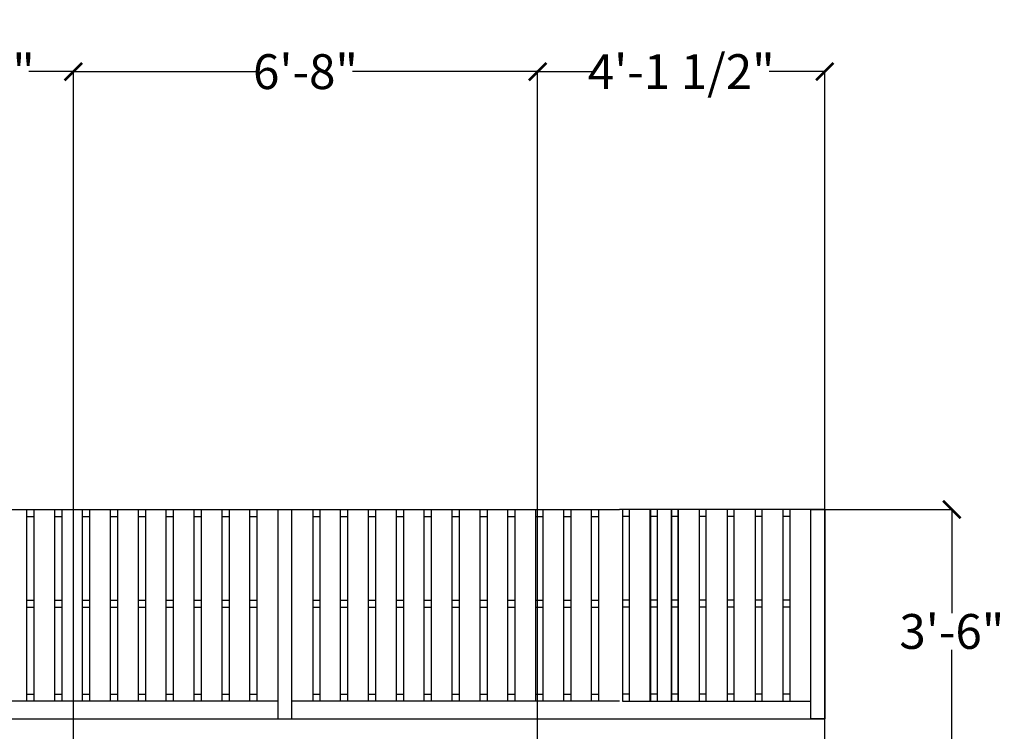
# Model space of a CAD drawing. Units: inches. Extents: x 2278 to 7495, y -71 to 1198.
# Tile 38 of 44: x 5007 to 5177, y 248 to 371. Entities that reach past the tile are written whole.
import ezdxf

# ---------------------------------------------------------------- set-up
doc = ezdxf.new("R2010")
doc.units = ezdxf.units.IN
doc.header["$MEASUREMENT"] = 0
for name, color, linetype, lineweight in [('A-ANNO-DIMS', 2, 'Continuous', 18), ('A-ANNO-TEXT', 7, 'Continuous', 25), ('A-ELEV', 7, 'Continuous', 25)]:
    doc.layers.add(name, color=color, linetype=linetype, lineweight=lineweight)
doc.styles.add('ATTR', font='romans.shx', dxfattribs={"width": 0.8, "height": 0.7})
doc.styles.get("Standard").update_dxf_attribs({"font": 'arial.ttf'})
doc.dimstyles.get("Standard").update_dxf_attribs({"dimtxt": 6, "dimasz": 3, "dimexe": 0.18, "dimexo": 0.0625, "dimgap": 0.09, "dimtad": 0, "dimtih": 1, "dimtoh": 1, "dimdec": 0, "dimzin": 0, "dimdsep": 46, "dimlunit": 3, "dimtxsty": 'Standard', "dimblk": 'ARCHTICK', "dimcen": 0.09, "dimadec": 0, "dimazin": 0, "dimtfac": 1, "dimtdec": 0, "dimtofl": 0, "dimtmove": 0, "dimatfit": 3, "dimfxl": 1, "dimtolj": 1, "dimtzin": 0, "dimarcsym": 0})

# ---------------------------------------------------------------- blocks, each defined once
blk = doc.blocks.new('Fence 2 EV')
for p, q in [((0, 60), (0, 0)), ((0.001, 60.008), (98.001, 60.008)), ((4, 0.002), (4, 60)), ((10, 60), (10, 5.002)), ((12, 60), (12, 5.002)), ((18, 5.002), (18, 60)), ((20, 60), (20, 5.002)), ((25.999, 5.002), (25.999, 60)), ((27.999, 60), (27.999, 5.002)), ((33.999, 5.002), (33.999, 60)), ((35.999, 60), (35.999, 5.002)), ((41.999, 5.002), (41.999, 60)), ((43.999, 60), (43.999, 5.002)), ((49.999, 5.002), (49.999, 60)), ((51.998, 60), (51.998, 5.002)), ((57.998, 5.002), (57.998, 60)), ((59.998, 60), (59.998, 5.002)), ((65.998, 5.002), (65.998, 60)), ((67.998, 60), (67.998, 5.002)), ((73.998, 5.002), (73.998, 60)), ((75.997, 60), (75.997, 5.002)), ((81.997, 5.002), (81.997, 60)), ((83.997, 60), (83.997, 5.002)), ((89.997, 5.002), (89.997, 60)), ((91.997, 60), (91.997, 5.002)), ((10, 58), (12, 58)), ((18, 58), (20, 58)), ((25.999, 58), (27.999, 58)), ((33.999, 58), (35.999, 58)), ((41.999, 58), (43.999, 58)), ((49.999, 58), (51.998, 58)), ((57.998, 58), (59.998, 58)), ((65.998, 58), (67.998, 58)), ((73.998, 58), (75.997, 58)), ((81.997, 58), (83.997, 58)), ((89.997, 58), (91.997, 58)), ((10, 34.001), (12, 34.001)), ((18, 34.001), (20, 34.001)), ((25.999, 34.001), (27.999, 34.001)), ((33.999, 34.001), (35.999, 34.001)), ((41.999, 34.001), (43.999, 34.001)), ((49.999, 34.001), (51.998, 34.001)), ((57.998, 34.001), (59.998, 34.001)), ((65.998, 34.001), (67.998, 34.001)), ((73.998, 34.001), (75.997, 34.001)), ((81.997, 34.001), (83.997, 34.001)), ((89.997, 34.001), (91.997, 34.001)), ((10, 32.001), (12, 32.001)), ((18, 32.001), (20, 32.001)), ((25.999, 32.001), (27.999, 32.001)), ((33.999, 32.001), (35.999, 32.001)), ((41.999, 32.001), (43.999, 32.001)), ((49.999, 32.001), (51.998, 32.001)), ((57.998, 32.001), (59.998, 32.001)), ((65.998, 32.001), (67.998, 32.001)), ((73.998, 32.001), (75.997, 32.001)), ((81.997, 32.001), (83.997, 32.001)), ((89.997, 32.001), (91.997, 32.001)), ((10, 7.002), (12, 7.002)), ((18, 7.002), (20, 7.002)), ((25.999, 7.002), (27.999, 7.002)), ((33.999, 7.002), (35.999, 7.002)), ((41.999, 7.002), (43.999, 7.002)), ((49.999, 7.002), (51.998, 7.002)), ((57.998, 7.002), (59.998, 7.002)), ((65.998, 7.002), (67.998, 7.002)), ((73.998, 7.002), (75.997, 7.002)), ((81.997, 7.002), (83.997, 7.002)), ((89.997, 7.002), (91.997, 7.002)), ((97.997, 5.002), (4, 5.002)), ((0, 0.002), (4, 0.002))]:
    blk.add_line(p, q)
at = {"style": 'ATTR', "width": 0.8, "flags": 9}
blk.add_attdef('ESTCODE', (0, 0), '', height=0.0196, dxfattribs=at)
blk = doc.blocks.new('_ArchTick')
at = {"color": 0, "linetype": 'ByBlock', "const_width": 0.15}
blk.add_lwpolyline([(-0.5, -0.5), (0.5, 0.5)], dxfattribs=at)
blk = doc.blocks.new('*D57')
at = {"layer": 'A-ANNO-DIMS', "color": 0, "lineweight": -2, "transparency": 16777216}
for p, q in [((4874.68, 250.19), (4874.68, 241.24)), ((4933.56, 250.19), (4933.56, 241.24)), ((4874.68, 241.42), (4933.56, 241.42)), ((4933.56, 241.42), (4936.56, 241.42))]:
    blk.add_line(p, q, dxfattribs=at)
at = {"layer": 'Defpoints', "color": 0, "transparency": 16777216}
for p in [(4874.68, 250.25), (4933.56, 250.25), (4933.56, 241.42)]:
    blk.add_point(p, dxfattribs=at)
at = {"layer": 'A-ANNO-DIMS', "color": 0, "lineweight": -2, "transparency": 16777216, "xscale": 3, "yscale": 3, "zscale": 3, "rotation": 180}
blk.add_blockref('_ArchTick', (4874.68, 241.42), dxfattribs=at)
at = {"layer": 'A-ANNO-DIMS', "color": 0, "lineweight": -2, "transparency": 16777216, "xscale": 3, "yscale": 3, "zscale": 3}
blk.add_blockref('_ArchTick', (4933.56, 241.42), dxfattribs=at)
at = {"layer": 'A-ANNO-DIMS', "color": 0, "transparency": 16777216, "insert": (4995.78, 241.42), "char_height": 6, "attachment_point": 5}
blk.add_mtext('\\A1;PARAPET RAILING 4\'-11" TYP.', dxfattribs=at)
blk = doc.blocks.new('*D123')
at = {"layer": 'A-ANNO-DIMS', "color": 0, "lineweight": -2, "transparency": 16777216}
for p, q in [((4736.95, 340.16), (4736.95, -23.43)), ((5145.68, -1.81), (5145.68, -23.43)), ((4736.95, -23.25), (4923.93, -23.25)), ((5145.68, -23.25), (4958.7, -23.25))]:
    blk.add_line(p, q, dxfattribs=at)
at = {"layer": 'Defpoints', "color": 0, "transparency": 16777216}
for p in [(4736.95, 340.22), (5145.68, -1.75), (5145.68, -23.25)]:
    blk.add_point(p, dxfattribs=at)
at = {"layer": 'A-ANNO-DIMS', "color": 0, "lineweight": -2, "transparency": 16777216, "xscale": 3, "yscale": 3, "zscale": 3, "rotation": 180}
blk.add_blockref('_ArchTick', (4736.95, -23.25), dxfattribs=at)
at = {"layer": 'A-ANNO-DIMS', "color": 0, "lineweight": -2, "transparency": 16777216, "xscale": 3, "yscale": 3, "zscale": 3}
blk.add_blockref('_ArchTick', (5145.68, -23.25), dxfattribs=at)
at = {"layer": 'A-ANNO-DIMS', "color": 0, "transparency": 16777216, "insert": (4941.31, -23.25), "char_height": 6, "attachment_point": 5}
blk.add_mtext('\\A1;34\'-0 1/2"', dxfattribs=at)
blk = doc.blocks.new('*D129')
at = {"layer": 'A-ANNO-DIMS', "color": 0, "lineweight": -2, "transparency": 16777216}
for p, q in [((4970.68, 60.78), (4970.68, 361.9)), ((4970.68, 361.72), (4978.37, 361.72)), ((5016.18, 361.72), (5008.48, 361.72)), ((5016.18, 99.32), (5016.18, 361.9))]:
    blk.add_line(p, q, dxfattribs=at)
at = {"layer": 'Defpoints', "color": 0, "transparency": 16777216}
for p in [(5016.18, 361.72), (5016.18, 99.25), (4970.68, 60.72)]:
    blk.add_point(p, dxfattribs=at)
at = {"layer": 'A-ANNO-DIMS', "color": 0, "lineweight": -2, "transparency": 16777216, "xscale": 3, "yscale": 3, "zscale": 3, "rotation": 180}
blk.add_blockref('_ArchTick', (4970.68, 361.72), dxfattribs=at)
at = {"layer": 'A-ANNO-DIMS', "color": 0, "lineweight": -2, "transparency": 16777216, "xscale": 3, "yscale": 3, "zscale": 3}
blk.add_blockref('_ArchTick', (5016.18, 361.72), dxfattribs=at)
at = {"layer": 'A-ANNO-DIMS', "color": 0, "transparency": 16777216, "insert": (4993.43, 361.72), "char_height": 6, "attachment_point": 5}
blk.add_mtext('\\A1;3\'-9 1/2"', dxfattribs=at)
blk = doc.blocks.new('*D130')
at = {"layer": 'A-ANNO-DIMS', "color": 0, "lineweight": -2, "transparency": 16777216}
for p, q in [((5016.18, 99.32), (5016.18, 361.9)), ((5016.18, 361.72), (5048.1, 361.72)), ((5096.18, 361.72), (5064.26, 361.72)), ((5096.18, 99.32), (5096.18, 361.9))]:
    blk.add_line(p, q, dxfattribs=at)
at = {"layer": 'Defpoints', "color": 0, "transparency": 16777216}
for p in [(5096.18, 361.72), (5016.18, 99.25), (5096.18, 99.25)]:
    blk.add_point(p, dxfattribs=at)
at = {"layer": 'A-ANNO-DIMS', "color": 0, "lineweight": -2, "transparency": 16777216, "xscale": 3, "yscale": 3, "zscale": 3, "rotation": 180}
blk.add_blockref('_ArchTick', (5016.18, 361.72), dxfattribs=at)
at = {"layer": 'A-ANNO-DIMS', "color": 0, "lineweight": -2, "transparency": 16777216, "xscale": 3, "yscale": 3, "zscale": 3}
blk.add_blockref('_ArchTick', (5096.18, 361.72), dxfattribs=at)
at = {"layer": 'A-ANNO-DIMS', "color": 0, "transparency": 16777216, "insert": (5056.18, 361.72), "char_height": 6, "attachment_point": 5}
blk.add_mtext('\\A1;6\'-8"', dxfattribs=at)
blk = doc.blocks.new('*D131')
at = {"layer": 'A-ANNO-DIMS', "color": 0, "lineweight": -2, "transparency": 16777216}
for p, q in [((5096.18, 99.32), (5096.18, 361.9)), ((5096.18, 361.72), (5105.75, 361.72)), ((5145.68, 361.72), (5136.1, 361.72)), ((5145.68, 118.32), (5145.68, 361.9))]:
    blk.add_line(p, q, dxfattribs=at)
at = {"layer": 'Defpoints', "color": 0, "transparency": 16777216}
for p in [(5145.68, 361.72), (5145.68, 118.25), (5096.18, 99.25)]:
    blk.add_point(p, dxfattribs=at)
at = {"layer": 'A-ANNO-DIMS', "color": 0, "lineweight": -2, "transparency": 16777216, "xscale": 3, "yscale": 3, "zscale": 3, "rotation": 180}
blk.add_blockref('_ArchTick', (5096.18, 361.72), dxfattribs=at)
at = {"layer": 'A-ANNO-DIMS', "color": 0, "lineweight": -2, "transparency": 16777216, "xscale": 3, "yscale": 3, "zscale": 3}
blk.add_blockref('_ArchTick', (5145.68, 361.72), dxfattribs=at)
at = {"layer": 'A-ANNO-DIMS', "color": 0, "transparency": 16777216, "insert": (5120.93, 361.72), "char_height": 6, "attachment_point": 5}
blk.add_mtext('\\A1;4\'-1 1/2"', dxfattribs=at)
blk = doc.blocks.new('*D142')
at = {"layer": 'A-ANNO-DIMS', "color": 0, "lineweight": -2, "transparency": 16777216}
for p, q in [((5143.34, 286.3), (5167.75, 286.3)), ((5167.57, 286.3), (5167.57, 268.43)), ((5167.57, 244.25), (5167.57, 262.12)), ((5145.74, 244.25), (5167.75, 244.25))]:
    blk.add_line(p, q, dxfattribs=at)
at = {"layer": 'Defpoints', "color": 0, "transparency": 16777216}
for p in [(5143.27, 286.3), (5167.57, 286.3), (5145.68, 244.25)]:
    blk.add_point(p, dxfattribs=at)
at = {"layer": 'A-ANNO-DIMS', "color": 0, "lineweight": -2, "transparency": 16777216, "xscale": 3, "yscale": 3, "zscale": 3}
for p, rotation in [((5167.57, 286.3), 90), ((5167.57, 244.25), 270)]:
    blk.add_blockref('_ArchTick', p, dxfattribs=dict(at, rotation=rotation))
at = {"layer": 'A-ANNO-DIMS', "color": 0, "transparency": 16777216, "insert": (5167.57, 265.28), "char_height": 6, "attachment_point": 5}
blk.add_mtext('\\A1;3\'-6"', dxfattribs=at)

msp = doc.modelspace()

# ---------------------------------------------------------------- linework, layer by layer
at = {"layer": 'A-ELEV'}
for p, q in [((5110.82, 286.3), (5110.3, 286.31)), ((5145.68, 286.31), (5110.82, 286.31)), ((5110.82, 286.3), (5110.82, 253.26)), ((5112.02, 285.1), (5110.82, 285.1)), ((5112.02, 253.26), (5112.02, 286.3)), ((5115.6, 253.26), (5115.6, 286.3)), ((5115.64, 285.1), (5115.6, 285.1)), ((5115.63, 286.3), (5115.63, 253.26)), ((5116.83, 285.1), (5115.63, 285.1)), ((5115.64, 253.26), (5115.64, 286.3)), ((5116.83, 253.26), (5116.83, 286.3)), ((5119.21, 286.3), (5119.21, 253.26)), ((5120.41, 285.1), (5119.21, 285.1)), ((5119.24, 286.3), (5119.24, 253.26)), ((5120.44, 285.1), (5119.24, 285.1)), ((5120.41, 253.26), (5120.41, 286.3)), ((5120.44, 253.26), (5120.44, 286.3)), ((5124.01, 286.3), (5124.01, 253.26)), ((5125.22, 285.1), (5124.01, 285.1)), ((5124.05, 286.3), (5124.05, 253.26)), ((5125.25, 285.1), (5124.05, 285.1)), ((5125.22, 253.26), (5125.22, 286.3)), ((5125.25, 253.26), (5125.25, 286.3)), ((5128.85, 286.3), (5128.85, 253.26)), ((5130.06, 285.1), (5128.85, 285.1)), ((5130.06, 253.26), (5130.06, 286.3)), ((5133.66, 286.3), (5133.66, 253.26)), ((5134.86, 285.1), (5133.66, 285.1)), ((5134.86, 253.26), (5134.86, 286.3)), ((5138.47, 286.3), (5138.47, 253.26)), ((5139.67, 285.1), (5138.47, 285.1)), ((5139.67, 286.3), (5139.67, 253.26)), ((5143.27, 250.25), (5143.27, 286.3)), ((5145.68, 286.3), (5145.68, 250.25)), ((5112.02, 270.68), (5110.82, 270.68)), ((5116.83, 270.68), (5115.63, 270.68)), ((5120.41, 270.68), (5119.21, 270.68)), ((5120.44, 270.68), (5119.24, 270.68)), ((5125.22, 270.68), (5124.01, 270.68)), ((5125.25, 270.68), (5124.05, 270.68)), ((5130.06, 270.68), (5128.85, 270.68)), ((5134.86, 270.68), (5133.66, 270.68)), ((5139.67, 270.68), (5138.47, 270.68)), ((5112.02, 269.48), (5110.82, 269.48)), ((5116.83, 269.48), (5115.63, 269.48)), ((5120.41, 269.48), (5119.21, 269.48)), ((5120.44, 269.48), (5119.24, 269.48)), ((5125.22, 269.48), (5124.01, 269.48)), ((5125.25, 269.48), (5124.05, 269.48)), ((5130.06, 269.48), (5128.85, 269.48)), ((5134.86, 269.48), (5133.66, 269.48)), ((5139.67, 269.48), (5138.47, 269.48)), ((5112.02, 254.46), (5110.82, 254.46)), ((5110.82, 253.26), (5143.27, 253.26)), ((5116.83, 254.46), (5115.63, 254.46)), ((5120.41, 254.46), (5119.21, 254.46)), ((5120.44, 254.46), (5119.24, 254.46)), ((5125.22, 254.46), (5124.01, 254.46)), ((5125.25, 254.46), (5124.05, 254.46)), ((5130.06, 254.46), (5128.85, 254.46)), ((5134.86, 254.46), (5133.66, 254.46)), ((5139.67, 254.46), (5138.47, 254.46)), ((4874.68, 250.25), (5145.68, 250.25)), ((5145.68, 250.25), (5143.27, 250.25)), ((5145.68, 164.45), (5145.68, 250.25))]:
    msp.add_line(p, q, dxfattribs=at)

# ---------------------------------------------------------------- block references
at = {"layer": 'A-ELEV', "xscale": 0.600830084310023, "yscale": 0.600830084310023, "zscale": 0.600830084310023}
for p in [(4992.54, 250.25), (5051.42, 250.25)]:
    msp.add_blockref('Fence 2 EV', p, dxfattribs=at)

# ---------------------------------------------------------------- texts
at = {"layer": 'A-ANNO-TEXT', "style": 'ATTR', "width": 0.8, "flags": 9}
msp.add_attdef('ESTCODE', (5145.68, 250.25), '', height=0.0118, dxfattribs=at)

# ---------------------------------------------------------------- dimensions: what is measured, and where the dimension line sits
at = {"layer": 'A-ANNO-DIMS'}
for base, p1, p2, picture, middle in [((5016.18, 361.72), (4970.68, 60.72), (5016.18, 99.25), '*D129', (4993.43, 361.72)), ((5145.68, 361.72), (5096.18, 99.25), (5145.68, 118.25), '*D131', (5120.93, 361.72)), ((5096.18, 361.72), (5016.18, 99.25), (5096.18, 99.25), '*D130', (5056.18, 361.72)), ((5145.68, -23.25), (4736.95, 340.22), (5145.68, -1.75), '*D123', (4941.31, -23.25))]:
    dim = msp.add_linear_dim(base=base, p1=p1, p2=p2, dimstyle='Standard', override={"dimdec": 1, "dimlfac": 1, "dimrnd": 0, "dimzin": 1, "dimdsep": 46, "dimlunit": 4, "dimfrac": 2}, dxfattribs=at)
    dim.commit()
    dim.dimension.update_dxf_attribs({"geometry": picture, "text_midpoint": middle})
dim = msp.add_linear_dim(base=(5167.5738, 286.3026), p1=(5145.6762, 244.2528), p2=(5143.2729, 286.3026), angle=90, dimstyle='Standard', override={"dimdec": 1, "dimlfac": 1, "dimrnd": 0, "dimzin": 1, "dimdsep": 46, "dimlunit": 4, "dimfrac": 2}, dxfattribs=at)
dim.commit()
dim.dimension.update_dxf_attribs({"geometry": '*D142', "text_midpoint": (5167.5738, 265.2777)})
dim = msp.add_linear_dim(base=(4933.56, 241.42), p1=(4874.68, 250.25), p2=(4933.56, 250.25), text='PARAPET RAILING <> TYP.', dimstyle='Standard', override={"dimdec": 1, "dimrnd": 0, "dimzin": 1, "dimlunit": 4, "dimfrac": 2}, dxfattribs=at)
dim.commit()
dim.dimension.update_dxf_attribs({"geometry": '*D57', "text_midpoint": (4995.78, 241.42)})

doc.saveas('drawing.dxf')
